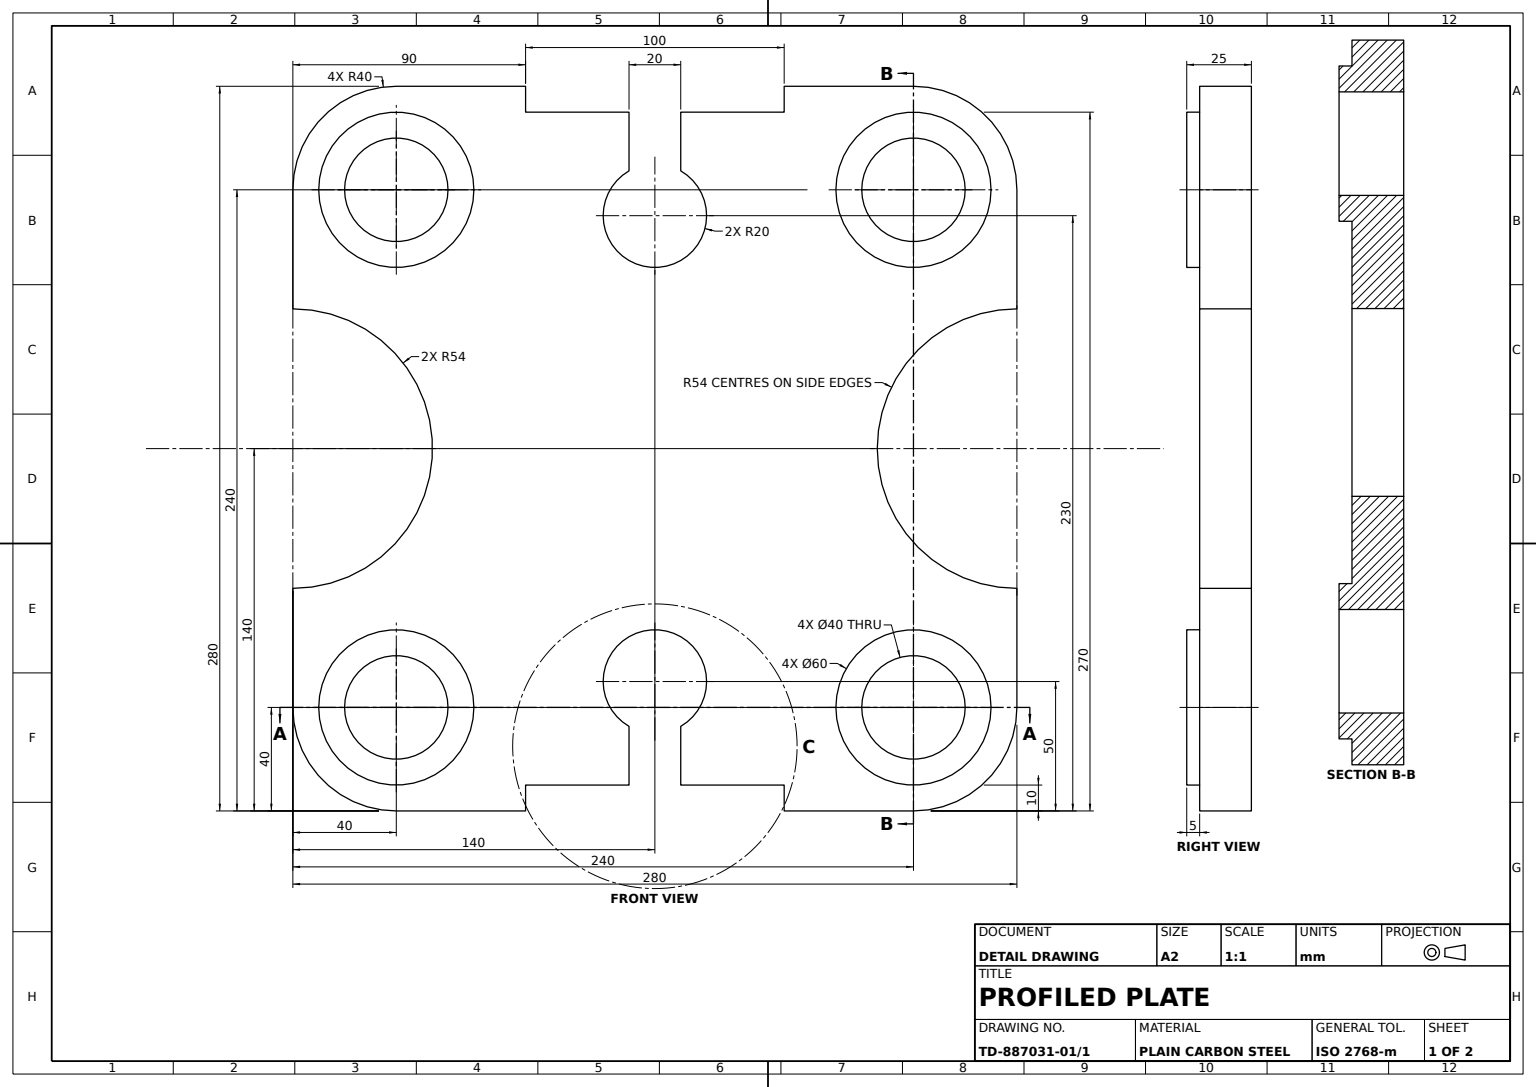
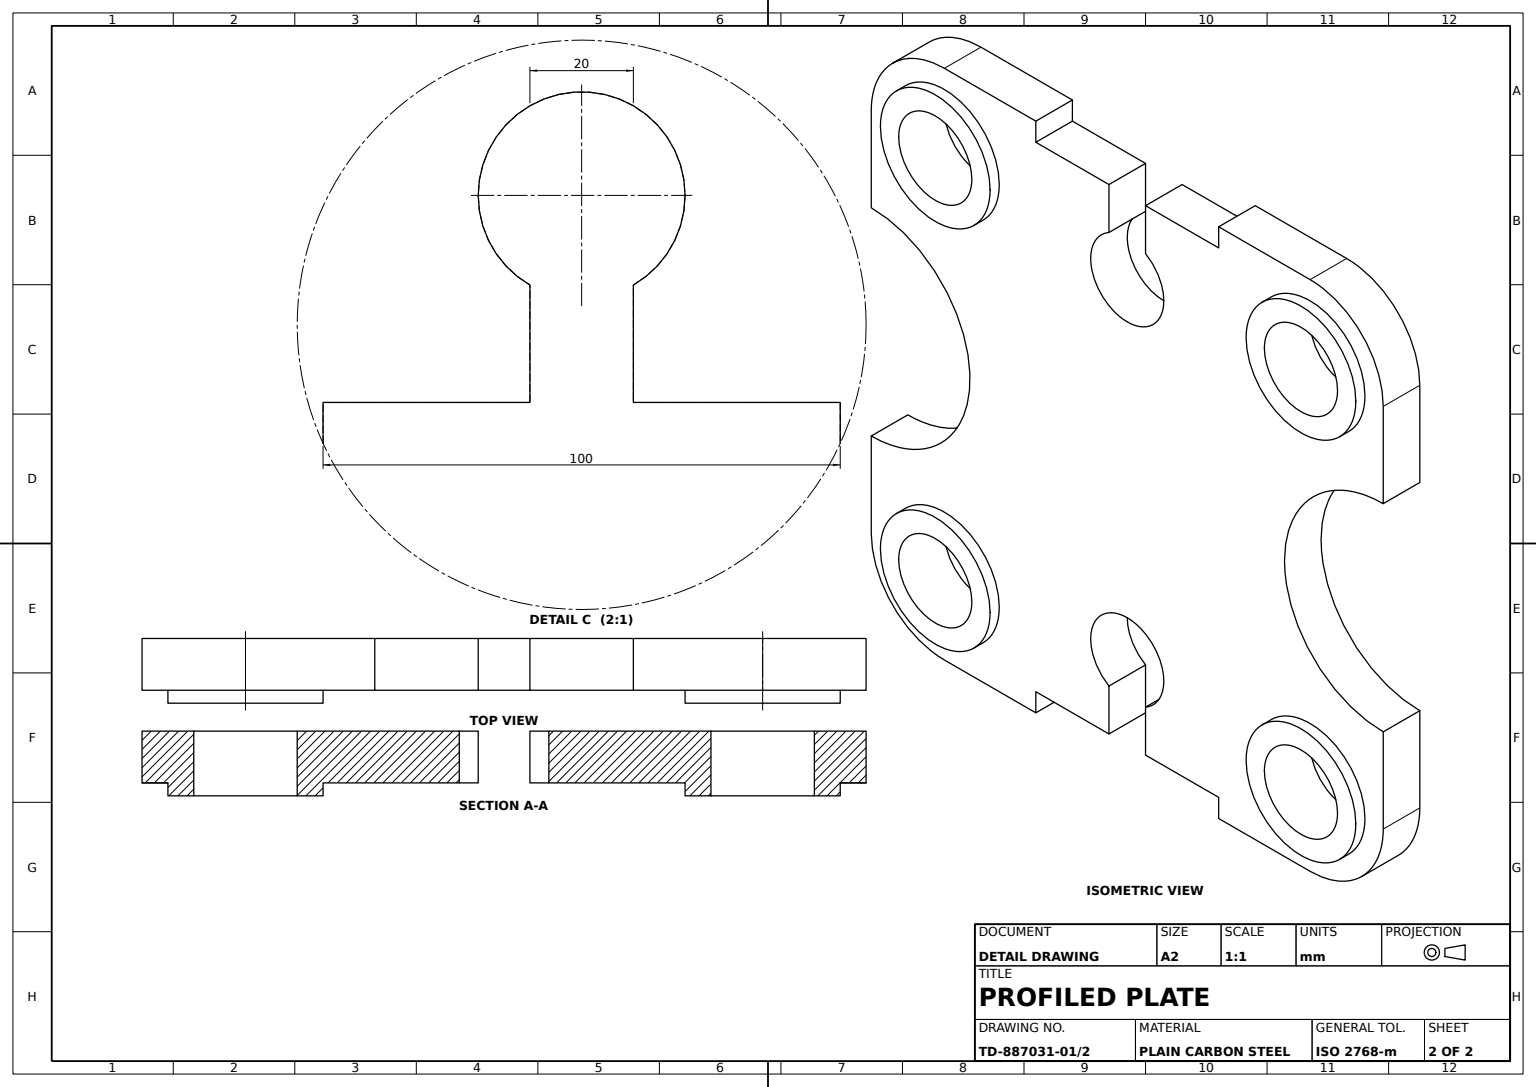
from build123d import *

# Parameters (mm, degrees)
BASE_PLATE_20MM_DEPTH          = 20
MOUNTING_BOSS_RINGS_SKETCH_R   = 30
MOUNTING_BOSS_RINGS_SKETCH_R_2 = 20
MOUNTING_BOSSES_4X_60_DEPTH    = 5
TOP_NOTCH_SKETCH_R             = 20
TOP_NOTCH_CUT_DEPTH            = 397.484552032


with BuildPart() as part:
    # Plate Profile Sketch → Base Plate 20mm (new body)
    with BuildSketch(Plane.XY):
        with BuildLine():
            Line((40, 0), (90, 0))
            Line((90, 0), (90, 10))
            Line((90, 10), (130, 10))
            Line((130, 10), (130, 32.679491924))
            ThreePointArc((130, 32.679491924), (140, 70), (150, 32.679491924))
            Line((150, 32.679491924), (150, 10))
            Line((150, 10), (190, 10))
            Line((190, 10), (190, 0))
            Line((190, 0), (240, 0))
            ThreePointArc((240, 0), (268.284271247, 11.715728753), (280, 40))
            Line((280, 40), (280, 86))
            ThreePointArc((280, 86), (226, 140), (280, 194))
            Line((280, 194), (280, 240))
            ThreePointArc((280, 240), (268.284271247, 268.284271247), (240, 280))
            Line((240, 280), (190, 280))
            Line((190, 280), (190, 270))
            Line((190, 270), (150, 270))
            Line((150, 270), (150, 247.320508076))
            ThreePointArc((150, 247.320508076), (140, 210), (130, 247.320508076))
            Line((130, 247.320508076), (130, 270))
            Line((130, 270), (90, 270))
            Line((90, 270), (90, 280))
            Line((90, 280), (40, 280))
            ThreePointArc((40, 280), (11.715728753, 268.284271247), (0, 240))
            Line((0, 240), (0, 194))
            ThreePointArc((0, 194), (54, 140), (0, 86))
            Line((0, 86), (0, 40))
            ThreePointArc((0, 40), (11.715728753, 11.715728753), (40, 0))
        make_face()
    extrude(amount=BASE_PLATE_20MM_DEPTH)

    # Mounting Boss Rings Sketch → Mounting Bosses 4xØ60 (add)
    # profile 1 of 4: a face of its own
    with BuildSketch(Plane.XY.offset(20)):
        with Locations((240, 240)):
            Circle(MOUNTING_BOSS_RINGS_SKETCH_R)
        with Locations((240, 240)):
            Circle(MOUNTING_BOSS_RINGS_SKETCH_R_2, mode=Mode.SUBTRACT)
    # profile 2 of 4: a face of its own
    with BuildSketch(Plane.XY.offset(20)):
        with Locations((40, 240)):
            Circle(MOUNTING_BOSS_RINGS_SKETCH_R)
        with Locations((40, 240)):
            Circle(MOUNTING_BOSS_RINGS_SKETCH_R_2, mode=Mode.SUBTRACT)
    # profile 3 of 4: a face of its own
    with BuildSketch(Plane.XY.offset(20)):
        with Locations((240, 40)):
            Circle(MOUNTING_BOSS_RINGS_SKETCH_R)
        with Locations((240, 40)):
            Circle(MOUNTING_BOSS_RINGS_SKETCH_R_2, mode=Mode.SUBTRACT)
    # profile 4 of 4: a face of its own
    with BuildSketch(Plane.XY.offset(20)):
        with Locations((40, 40)):
            Circle(MOUNTING_BOSS_RINGS_SKETCH_R)
        with Locations((40, 40)):
            Circle(MOUNTING_BOSS_RINGS_SKETCH_R_2, mode=Mode.SUBTRACT)
    extrude(amount=MOUNTING_BOSSES_4X_60_DEPTH)

    # Top Notch Sketch → Top Notch Cut (cut, through all)
    with BuildSketch(Plane.XY.offset(20)):
        with Locations((40, 240)):
            Circle(TOP_NOTCH_SKETCH_R)
        with Locations((240, 240)):
            Circle(TOP_NOTCH_SKETCH_R)
        with Locations((240, 40)):
            Circle(TOP_NOTCH_SKETCH_R)
        with Locations((40, 40)):
            Circle(TOP_NOTCH_SKETCH_R)
    extrude(amount=-TOP_NOTCH_CUT_DEPTH, mode=Mode.SUBTRACT)


solid = part.part
